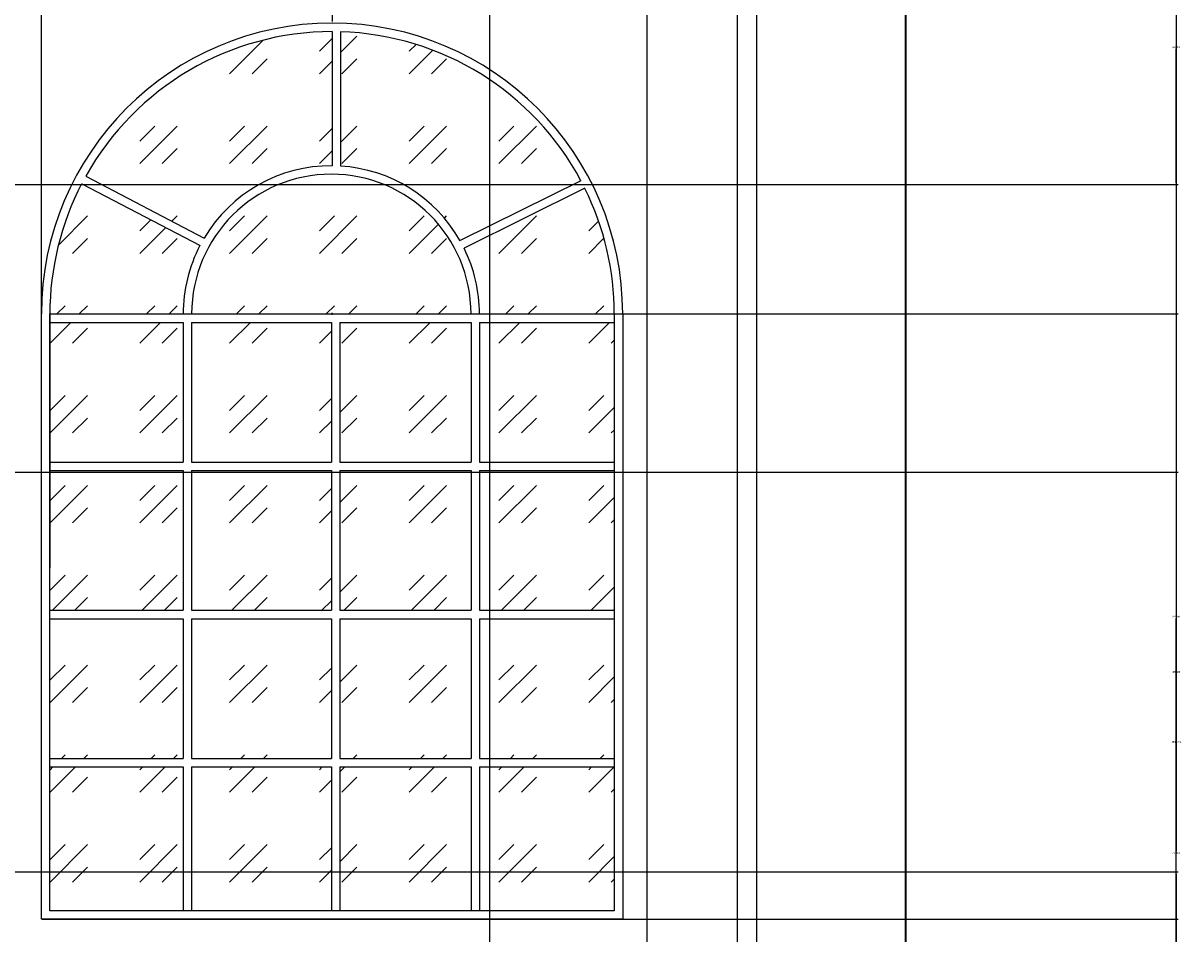
# Model space of a CAD drawing. Units: inches. Extents: x 93 to 565, y 123 to 656.
# Tile 12 of 18: x 456 to 565, y 377 to 463. Entities that reach past the tile are written whole.
import ezdxf

# ---------------------------------------------------------------- set-up
doc = ezdxf.new("R2010")
doc.units = ezdxf.units.IN
doc.header["$MEASUREMENT"] = 0
for name, color, linetype, lineweight in [('A-ANNO-DIMS', 2, 'Continuous', 18), ('A-ELEV', 7, 'Continuous', 35), ('A-GLAZ', 4, 'Continuous', 25)]:
    doc.layers.add(name, color=color, linetype=linetype, lineweight=lineweight)
doc.styles.get("Standard").update_dxf_attribs({"font": 'arial.ttf'})
doc.dimstyles.get("Standard").update_dxf_attribs({"dimtxt": 0.18, "dimasz": 0.18, "dimexe": 0.18, "dimexo": 0.0625, "dimgap": 0.09, "dimtad": 0, "dimtih": 1, "dimtoh": 1, "dimdec": 4, "dimzin": 0, "dimdsep": 46, "dimtxsty": 'Standard', "dimcen": 0.09, "dimadec": 0, "dimazin": 0, "dimtfac": 1, "dimtdec": 4, "dimtofl": 0, "dimtmove": 0, "dimatfit": 3, "dimfxl": 1, "dimtolj": 1, "dimtzin": 0, "dimarcsym": 0})

# ---------------------------------------------------------------- blocks, each defined once
blk = doc.blocks.new('WIN-ARCHED')
for p, q in [((26.67, 83.05), (26.67, 70.38)), ((27.47, 83.04), (27.47, 70.36)), ((3.39, 69.39), (14.58, 63.55)), ((50.18, 68.96), (38.77, 63.31)), ((3.01, 68.68), (14.19, 62.86)), ((50.55, 68.25), (39.15, 62.6)), ((0, 56.38), (12.6, 56.38)), ((0, 56.38), (0.2, 56.38)), ((0, 56.38), (0, 32.38)), ((13.4, 56.38), (39.8, 56.38)), ((40.6, 56.38), (53.33, 56.38)), ((0, 55.58), (12.6, 55.58)), ((12.6, 55.58), (12.6, 42.38)), ((13.4, 55.58), (13.4, 42.38)), ((13.4, 55.58), (26.6, 55.58)), ((26.6, 55.58), (26.6, 42.38)), ((27.4, 55.58), (27.4, 42.38)), ((27.4, 55.58), (39.8, 55.58)), ((39.8, 55.58), (39.8, 42.38)), ((40.6, 55.58), (40.6, 42.38)), ((40.6, 55.58), (53.33, 55.58)), ((0, 42.38), (12.6, 42.38)), ((0, 41.58), (12.6, 41.58)), ((12.6, 41.58), (12.6, 28.38)), ((13.4, 42.38), (26.6, 42.38)), ((13.4, 41.58), (13.4, 28.38)), ((13.4, 41.58), (26.6, 41.58)), ((26.6, 41.58), (26.6, 28.38)), ((27.4, 42.38), (39.8, 42.38)), ((27.4, 41.58), (27.4, 28.38)), ((27.4, 41.58), (39.8, 41.58)), ((39.8, 41.58), (39.8, 28.38)), ((40.6, 42.38), (53.33, 42.38)), ((40.6, 41.58), (40.6, 28.38)), ((40.6, 41.58), (53.33, 41.58)), ((0, 28.38), (12.6, 28.38)), ((0, 27.58), (12.6, 27.58)), ((12.6, 27.58), (12.6, 14.38)), ((13.4, 28.38), (26.6, 28.38)), ((13.4, 27.58), (13.4, 14.38)), ((13.4, 27.58), (26.6, 27.58)), ((26.6, 27.58), (26.6, 14.38)), ((27.4, 28.38), (39.8, 28.38)), ((27.4, 27.58), (27.4, 14.38)), ((27.4, 27.58), (39.8, 27.58)), ((39.8, 27.58), (39.8, 14.38)), ((40.6, 28.38), (53.33, 28.38)), ((40.6, 27.58), (40.6, 14.38)), ((40.6, 27.58), (53.33, 27.58)), ((0, 14.38), (12.6, 14.38)), ((13.4, 14.38), (26.6, 14.38)), ((27.4, 14.38), (39.8, 14.38)), ((40.6, 14.38), (53.33, 14.38)), ((0, 13.58), (12.6, 13.58)), ((12.6, 13.58), (12.6, 0)), ((13.4, 13.58), (13.4, 0)), ((13.4, 13.58), (26.6, 13.58)), ((26.6, 13.58), (26.6, 0)), ((27.4, 13.58), (27.4, 0)), ((27.4, 13.58), (39.8, 13.58)), ((39.8, 13.58), (39.8, 0)), ((40.6, 13.58), (40.6, 0)), ((40.6, 13.58), (53.33, 13.58))]:
    blk.add_line(p, q)
blk.add_lwpolyline([(53.33, 56.38), (53.33, 0), (0, 0), (0, 56.38)])
for centre, radius, start, end in [((26.67, 56.38), 26.67, 90, 150.8167), ((26.67, 56.38), 26.67, 28.1372, 88.2808), ((26.6, 56.38), 14, 89.7291, 149.1942), ((26.6, 56.38), 14, 29.6307, 86.4528), ((26.6, 56.38), 13.2, 0, 180), ((26.67, 56.38), 26.67, 152.5358, 180), ((26.67, 56.38), 26.67, 0, 26.418), ((26.6, 56.38), 14, 152.4701, 180), ((26.6, 56.38), 14, 0, 26.3549)]:
    blk.add_arc(centre, radius, start, end)
blk = doc.blocks.new('*D30')
at = {"layer": 'A-ANNO-DIMS', "color": 0, "lineweight": -2, "transparency": 16777216}
for p, q in [((437.19, 594.34), (437.19, 134)), ((539.08, 159.67), (539.08, 134)), ((437.37, 134.18), (487.75, 134.18)), ((538.9, 134.18), (488.52, 134.18))]:
    blk.add_line(p, q, dxfattribs=at)
at = {"layer": 'A-ANNO-DIMS', "color": 0, "transparency": 16777216}
for points in [[(437.37, 134.21), (437.37, 134.15), (437.19, 134.18)], [(538.9, 134.21), (538.9, 134.15), (539.08, 134.18)]]:
    blk.add_solid(points, dxfattribs=at)
at = {"layer": 'Defpoints', "color": 0, "transparency": 16777216}
for p in [(437.19, 594.4), (539.08, 159.73), (539.08, 134.18)]:
    blk.add_point(p, dxfattribs=at)
at = {"layer": 'A-ANNO-DIMS', "color": 0, "transparency": 16777216, "insert": (488.13, 134.18), "char_height": 0.18, "attachment_point": 5}
blk.add_mtext('\\A1;101.9', dxfattribs=at)
blk = doc.blocks.new('*D31')
at = {"layer": 'A-ANNO-DIMS', "color": 0, "lineweight": -2, "transparency": 16777216}
for p, q in [((417.87, 630.4), (564.81, 630.4)), ((564.63, 630.22), (564.63, 395.25)), ((564.63, 159.91), (564.63, 394.89)), ((119.14, 159.73), (564.81, 159.73))]:
    blk.add_line(p, q, dxfattribs=at)
at = {"layer": 'A-ANNO-DIMS', "color": 0, "transparency": 16777216}
for points in [[(564.6, 630.22), (564.66, 630.22), (564.63, 630.4)], [(564.6, 159.91), (564.66, 159.91), (564.63, 159.73)]]:
    blk.add_solid(points, dxfattribs=at)
at = {"layer": 'Defpoints', "color": 0, "transparency": 16777216}
for p in [(417.81, 630.4), (564.63, 630.4), (119.08, 159.73)]:
    blk.add_point(p, dxfattribs=at)
at = {"layer": 'A-ANNO-DIMS', "color": 0, "transparency": 16777216, "insert": (564.63, 395.07), "char_height": 0.18, "attachment_point": 5}
blk.add_mtext('\\A1;470.7', dxfattribs=at)
blk = doc.blocks.new('*D67')
at = {"layer": 'A-ANNO-DIMS', "color": 0, "lineweight": -2, "transparency": 16777216}
for p, q in [((331.87, 420.57), (564.81, 420.57)), ((564.63, 420.39), (564.63, 384.75)), ((564.63, 348.75), (564.63, 384.39)), ((331.87, 348.57), (564.81, 348.57))]:
    blk.add_line(p, q, dxfattribs=at)
at = {"layer": 'A-ANNO-DIMS', "color": 0, "transparency": 16777216}
for points in [[(564.6, 420.39), (564.66, 420.39), (564.63, 420.57)], [(564.6, 348.75), (564.66, 348.75), (564.63, 348.57)]]:
    blk.add_solid(points, dxfattribs=at)
at = {"layer": 'Defpoints', "color": 0, "transparency": 16777216}
for p in [(331.81, 420.57), (564.63, 420.57), (331.81, 348.57)]:
    blk.add_point(p, dxfattribs=at)
at = {"layer": 'A-ANNO-DIMS', "color": 0, "transparency": 16777216, "insert": (564.63, 384.57), "char_height": 0.18, "attachment_point": 5}
blk.add_mtext('\\A1;72', dxfattribs=at)
blk = doc.blocks.new('*D70')
at = {"layer": 'A-ANNO-DIMS', "color": 0, "lineweight": -2, "transparency": 16777216}
for p, q in [((428.68, 420.57), (564.81, 420.57)), ((564.63, 420.39), (564.63, 401.87)), ((564.63, 382.98), (564.63, 401.5)), ((428.68, 382.8), (564.81, 382.8))]:
    blk.add_line(p, q, dxfattribs=at)
at = {"layer": 'A-ANNO-DIMS', "color": 0, "transparency": 16777216}
for points in [[(564.6, 420.39), (564.66, 420.39), (564.63, 420.57)], [(564.6, 382.98), (564.66, 382.98), (564.63, 382.8)]]:
    blk.add_solid(points, dxfattribs=at)
at = {"layer": 'Defpoints', "color": 0, "transparency": 16777216}
for p in [(428.62, 420.57), (564.63, 420.57), (428.62, 382.8)]:
    blk.add_point(p, dxfattribs=at)
at = {"layer": 'A-ANNO-DIMS', "color": 0, "transparency": 16777216, "insert": (564.63, 401.68), "char_height": 0.18, "attachment_point": 5}
blk.add_mtext('\\A1;37.77', dxfattribs=at)
blk = doc.blocks.new('*D71')
at = {"layer": 'A-ANNO-DIMS', "color": 0, "lineweight": -2, "transparency": 16777216}
for p, q in [((428.68, 382.8), (564.81, 382.8)), ((564.63, 382.62), (564.63, 372.46)), ((564.63, 361.93), (564.63, 372.09)), ((437.25, 361.75), (564.81, 361.75))]:
    blk.add_line(p, q, dxfattribs=at)
at = {"layer": 'A-ANNO-DIMS', "color": 0, "transparency": 16777216}
for points in [[(564.6, 382.62), (564.66, 382.62), (564.63, 382.8)], [(564.6, 361.93), (564.66, 361.93), (564.63, 361.75)]]:
    blk.add_solid(points, dxfattribs=at)
at = {"layer": 'Defpoints', "color": 0, "transparency": 16777216}
for p in [(428.62, 382.8), (437.19, 361.75), (564.63, 361.75)]:
    blk.add_point(p, dxfattribs=at)
at = {"layer": 'A-ANNO-DIMS', "color": 0, "transparency": 16777216, "insert": (564.63, 372.27), "char_height": 0.18, "attachment_point": 5}
blk.add_mtext('\\A1;21.05', dxfattribs=at)
blk = doc.blocks.new('*D73')
at = {"layer": 'A-ANNO-DIMS', "color": 0, "lineweight": -2, "transparency": 16777216}
for p, q in [((437.25, 473.73), (564.81, 473.73)), ((564.63, 473.55), (564.63, 460.91)), ((564.63, 447.91), (564.63, 460.55)), ((437.25, 447.73), (564.81, 447.73))]:
    blk.add_line(p, q, dxfattribs=at)
at = {"layer": 'A-ANNO-DIMS', "color": 0, "transparency": 16777216}
for points in [[(564.6, 473.55), (564.66, 473.55), (564.63, 473.73)], [(564.6, 447.91), (564.66, 447.91), (564.63, 447.73)]]:
    blk.add_solid(points, dxfattribs=at)
at = {"layer": 'Defpoints', "color": 0, "transparency": 16777216}
for p in [(437.19, 473.73), (564.63, 473.73), (437.19, 447.73)]:
    blk.add_point(p, dxfattribs=at)
at = {"layer": 'A-ANNO-DIMS', "color": 0, "transparency": 16777216, "insert": (564.63, 460.73), "char_height": 0.18, "attachment_point": 5}
blk.add_mtext('\\A1;26', dxfattribs=at)
blk = doc.blocks.new('*D82')
at = {"layer": 'A-ANNO-DIMS', "color": 0, "lineweight": -2, "transparency": 16777216}
for p, q in [((437.19, 447.79), (437.19, 656.13)), ((437.37, 655.95), (446.83, 655.95)), ((457.21, 655.95), (447.76, 655.95)), ((457.39, 378.4), (457.39, 656.13))]:
    blk.add_line(p, q, dxfattribs=at)
at = {"layer": 'A-ANNO-DIMS', "color": 0, "transparency": 16777216}
for points in [[(437.37, 655.98), (437.37, 655.92), (437.19, 655.95)], [(457.21, 655.98), (457.21, 655.92), (457.39, 655.95)]]:
    blk.add_solid(points, dxfattribs=at)
at = {"layer": 'Defpoints', "color": 0, "transparency": 16777216}
for p in [(457.39, 655.95), (437.19, 447.73), (457.39, 378.34)]:
    blk.add_point(p, dxfattribs=at)
at = {"layer": 'A-ANNO-DIMS', "color": 0, "transparency": 16777216, "insert": (447.29, 655.95), "char_height": 0.18, "attachment_point": 5}
blk.add_mtext('\\A1;20.205', dxfattribs=at)
blk = doc.blocks.new('*D83')
at = {"layer": 'A-ANNO-DIMS', "color": 0, "lineweight": -2, "transparency": 16777216}
for p, q in [((457.46, 378.34), (564.81, 378.34)), ((564.63, 378.16), (564.63, 370.22)), ((564.63, 361.93), (564.63, 369.86)), ((437.25, 361.75), (564.81, 361.75))]:
    blk.add_line(p, q, dxfattribs=at)
at = {"layer": 'A-ANNO-DIMS', "color": 0, "transparency": 16777216}
for points in [[(564.6, 378.16), (564.66, 378.16), (564.63, 378.34)], [(564.6, 361.93), (564.66, 361.93), (564.63, 361.75)]]:
    blk.add_solid(points, dxfattribs=at)
at = {"layer": 'Defpoints', "color": 0, "transparency": 16777216}
for p in [(457.39, 378.34), (437.19, 361.75), (564.63, 361.75)]:
    blk.add_point(p, dxfattribs=at)
at = {"layer": 'A-ANNO-DIMS', "color": 0, "transparency": 16777216, "insert": (564.63, 370.04), "char_height": 0.18, "attachment_point": 5}
blk.add_mtext('\\A1;16.59', dxfattribs=at)
blk = doc.blocks.new('*D84')
at = {"layer": 'A-ANNO-DIMS', "color": 0, "lineweight": -2, "transparency": 16777216}
for p, q in [((458.26, 435.52), (564.81, 435.52)), ((564.63, 435.34), (564.63, 407.11)), ((564.63, 378.52), (564.63, 406.75)), ((457.46, 378.34), (564.81, 378.34))]:
    blk.add_line(p, q, dxfattribs=at)
at = {"layer": 'A-ANNO-DIMS', "color": 0, "transparency": 16777216}
for points in [[(564.6, 435.34), (564.66, 435.34), (564.63, 435.52)], [(564.6, 378.52), (564.66, 378.52), (564.63, 378.34)]]:
    blk.add_solid(points, dxfattribs=at)
at = {"layer": 'Defpoints', "color": 0, "transparency": 16777216}
for p in [(458.19, 435.52), (564.63, 435.52), (457.39, 378.34)]:
    blk.add_point(p, dxfattribs=at)
at = {"layer": 'A-ANNO-DIMS', "color": 0, "transparency": 16777216, "insert": (564.63, 406.93), "char_height": 0.18, "attachment_point": 5}
blk.add_mtext('\\A1;57.18', dxfattribs=at)
blk = doc.blocks.new('*D91')
at = {"layer": 'A-ANNO-DIMS', "color": 0, "lineweight": -2, "transparency": 16777216}
for p, q in [((499.73, 599.75), (499.73, 134)), ((437.19, 594.34), (437.19, 134)), ((437.37, 134.18), (468.07, 134.18)), ((499.55, 134.18), (468.85, 134.18))]:
    blk.add_line(p, q, dxfattribs=at)
at = {"layer": 'A-ANNO-DIMS', "color": 0, "transparency": 16777216}
for points in [[(437.37, 134.21), (437.37, 134.15), (437.19, 134.18)], [(499.55, 134.21), (499.55, 134.15), (499.73, 134.18)]]:
    blk.add_solid(points, dxfattribs=at)
at = {"layer": 'Defpoints', "color": 0, "transparency": 16777216}
for p in [(499.73, 599.82), (437.19, 594.4), (499.73, 134.18)]:
    blk.add_point(p, dxfattribs=at)
at = {"layer": 'A-ANNO-DIMS', "color": 0, "transparency": 16777216, "insert": (468.46, 134.18), "char_height": 0.18, "attachment_point": 5}
blk.add_mtext('\\A1;62.54', dxfattribs=at)
blk = doc.blocks.new('*D92')
at = {"layer": 'A-ANNO-DIMS', "color": 0, "lineweight": -2, "transparency": 16777216}
for p, q in [((523.14, 603.14), (523.14, 134)), ((499.73, 599.75), (499.73, 134)), ((499.91, 134.18), (510.97, 134.18)), ((522.96, 134.18), (511.9, 134.18))]:
    blk.add_line(p, q, dxfattribs=at)
at = {"layer": 'A-ANNO-DIMS', "color": 0, "transparency": 16777216}
for points in [[(499.91, 134.21), (499.91, 134.15), (499.73, 134.18)], [(522.96, 134.21), (522.96, 134.15), (523.14, 134.18)]]:
    blk.add_solid(points, dxfattribs=at)
at = {"layer": 'Defpoints', "color": 0, "transparency": 16777216}
for p in [(523.14, 603.2), (499.73, 599.82), (523.14, 134.18)]:
    blk.add_point(p, dxfattribs=at)
at = {"layer": 'A-ANNO-DIMS', "color": 0, "transparency": 16777216, "insert": (511.44, 134.18), "char_height": 0.18, "attachment_point": 5}
blk.add_mtext('\\A1;23.412', dxfattribs=at)
blk = doc.blocks.new('*D93')
at = {"layer": 'A-ANNO-DIMS', "color": 0, "lineweight": -2, "transparency": 16777216}
for p, q in [((523.14, 603.14), (523.14, 134)), ((539.08, 594.34), (539.08, 134)), ((523.32, 134.18), (530.66, 134.18)), ((538.9, 134.18), (531.57, 134.18))]:
    blk.add_line(p, q, dxfattribs=at)
at = {"layer": 'A-ANNO-DIMS', "color": 0, "transparency": 16777216}
for points in [[(523.32, 134.21), (523.32, 134.15), (523.14, 134.18)], [(538.9, 134.21), (538.9, 134.15), (539.08, 134.18)]]:
    blk.add_solid(points, dxfattribs=at)
at = {"layer": 'Defpoints', "color": 0, "transparency": 16777216}
for p in [(523.14, 603.2), (539.08, 594.4), (539.08, 134.18)]:
    blk.add_point(p, dxfattribs=at)
at = {"layer": 'A-ANNO-DIMS', "color": 0, "transparency": 16777216, "insert": (531.11, 134.18), "char_height": 0.18, "attachment_point": 5}
blk.add_mtext('\\A1;15.938', dxfattribs=at)
blk = doc.blocks.new('*D101')
at = {"layer": 'A-ANNO-DIMS', "color": 0, "lineweight": -2, "transparency": 16777216}
for p, q in [((485.04, 479.47), (484.86, 479.47)), ((484.86, 479.47), (484.86, 463.17)), ((484.77, 435.52), (484.95, 435.52)), ((484.86, 435.43), (484.86, 435.61))]:
    blk.add_line(p, q, dxfattribs=at)
at = {"layer": 'A-ANNO-DIMS', "color": 0, "transparency": 16777216}
blk.add_solid([(484.83, 463.17), (484.89, 463.17), (484.86, 462.99)], dxfattribs=at)
at = {"layer": 'Defpoints', "color": 0, "transparency": 16777216}
for p in [(484.86, 462.99), (484.86, 435.52)]:
    blk.add_point(p, dxfattribs=at)
at = {"layer": 'A-ANNO-DIMS', "color": 0, "transparency": 16777216, "insert": (485.78, 479.47), "char_height": 0.18, "attachment_point": 5}
blk.add_mtext('\\A1;2X R27.466', dxfattribs=at)
blk = doc.blocks.new('*D109')
at = {"layer": 'A-ANNO-DIMS', "color": 0, "lineweight": -2, "transparency": 16777216}
for p, q in [((437.19, 594.34), (437.19, 134)), ((539.08, 159.67), (539.08, 134)), ((437.37, 134.18), (487.63, 134.18)), ((538.9, 134.18), (488.64, 134.18))]:
    blk.add_line(p, q, dxfattribs=at)
at = {"layer": 'A-ANNO-DIMS', "color": 0, "transparency": 16777216}
for points in [[(437.37, 134.21), (437.37, 134.15), (437.19, 134.18)], [(538.9, 134.21), (538.9, 134.15), (539.08, 134.18)]]:
    blk.add_solid(points, dxfattribs=at)
at = {"layer": 'Defpoints', "color": 0, "transparency": 16777216}
for p in [(437.19, 594.4), (539.08, 159.73), (539.08, 134.18)]:
    blk.add_point(p, dxfattribs=at)
at = {"layer": 'A-ANNO-DIMS', "color": 0, "transparency": 16777216, "insert": (488.13, 134.18), "char_height": 0.18, "attachment_point": 5}
blk.add_mtext('\\A1;101.891', dxfattribs=at)
blk = doc.blocks.new('*D110')
at = {"layer": 'A-ANNO-DIMS', "color": 0, "lineweight": -2, "transparency": 16777216}
for p, q in [((417.87, 630.4), (564.81, 630.4)), ((564.63, 630.22), (564.63, 395.25)), ((564.63, 159.91), (564.63, 394.89)), ((119.14, 159.73), (564.81, 159.73))]:
    blk.add_line(p, q, dxfattribs=at)
at = {"layer": 'A-ANNO-DIMS', "color": 0, "transparency": 16777216}
for points in [[(564.6, 630.22), (564.66, 630.22), (564.63, 630.4)], [(564.6, 159.91), (564.66, 159.91), (564.63, 159.73)]]:
    blk.add_solid(points, dxfattribs=at)
at = {"layer": 'Defpoints', "color": 0, "transparency": 16777216}
for p in [(417.81, 630.4), (564.63, 630.4), (119.08, 159.73)]:
    blk.add_point(p, dxfattribs=at)
at = {"layer": 'A-ANNO-DIMS', "color": 0, "transparency": 16777216, "insert": (564.63, 395.07), "char_height": 0.18, "attachment_point": 5}
blk.add_mtext('\\A1;470.673', dxfattribs=at)
blk = doc.blocks.new('*D146')
at = {"layer": 'A-ANNO-DIMS', "color": 0, "lineweight": -2, "transparency": 16777216}
for p, q in [((331.87, 420.57), (564.81, 420.57)), ((564.63, 420.39), (564.63, 384.75)), ((564.63, 348.75), (564.63, 384.39)), ((331.87, 348.57), (564.81, 348.57))]:
    blk.add_line(p, q, dxfattribs=at)
at = {"layer": 'A-ANNO-DIMS', "color": 0, "transparency": 16777216}
for points in [[(564.6, 420.39), (564.66, 420.39), (564.63, 420.57)], [(564.6, 348.75), (564.66, 348.75), (564.63, 348.57)]]:
    blk.add_solid(points, dxfattribs=at)
at = {"layer": 'Defpoints', "color": 0, "transparency": 16777216}
for p in [(331.81, 420.57), (564.63, 420.57), (331.81, 348.57)]:
    blk.add_point(p, dxfattribs=at)
at = {"layer": 'A-ANNO-DIMS', "color": 0, "transparency": 16777216, "insert": (564.63, 384.57), "char_height": 0.18, "attachment_point": 5}
blk.add_mtext('\\A1;72.000', dxfattribs=at)
blk = doc.blocks.new('*D149')
at = {"layer": 'A-ANNO-DIMS', "color": 0, "lineweight": -2, "transparency": 16777216}
for p, q in [((428.68, 420.57), (564.81, 420.57)), ((564.63, 420.39), (564.63, 401.87)), ((564.63, 382.98), (564.63, 401.5)), ((428.68, 382.8), (564.81, 382.8))]:
    blk.add_line(p, q, dxfattribs=at)
at = {"layer": 'A-ANNO-DIMS', "color": 0, "transparency": 16777216}
for points in [[(564.6, 420.39), (564.66, 420.39), (564.63, 420.57)], [(564.6, 382.98), (564.66, 382.98), (564.63, 382.8)]]:
    blk.add_solid(points, dxfattribs=at)
at = {"layer": 'Defpoints', "color": 0, "transparency": 16777216}
for p in [(428.62, 420.57), (564.63, 420.57), (428.62, 382.8)]:
    blk.add_point(p, dxfattribs=at)
at = {"layer": 'A-ANNO-DIMS', "color": 0, "transparency": 16777216, "insert": (564.63, 401.68), "char_height": 0.18, "attachment_point": 5}
blk.add_mtext('\\A1;37.768', dxfattribs=at)
blk = doc.blocks.new('*D150')
at = {"layer": 'A-ANNO-DIMS', "color": 0, "lineweight": -2, "transparency": 16777216}
for p, q in [((428.68, 382.8), (564.81, 382.8)), ((564.63, 382.62), (564.63, 372.46)), ((564.63, 361.93), (564.63, 372.09)), ((437.25, 361.75), (564.81, 361.75))]:
    blk.add_line(p, q, dxfattribs=at)
at = {"layer": 'A-ANNO-DIMS', "color": 0, "transparency": 16777216}
for points in [[(564.6, 382.62), (564.66, 382.62), (564.63, 382.8)], [(564.6, 361.93), (564.66, 361.93), (564.63, 361.75)]]:
    blk.add_solid(points, dxfattribs=at)
at = {"layer": 'Defpoints', "color": 0, "transparency": 16777216}
for p in [(428.62, 382.8), (437.19, 361.75), (564.63, 361.75)]:
    blk.add_point(p, dxfattribs=at)
at = {"layer": 'A-ANNO-DIMS', "color": 0, "transparency": 16777216, "insert": (564.63, 372.27), "char_height": 0.18, "attachment_point": 5}
blk.add_mtext('\\A1;21.052', dxfattribs=at)
blk = doc.blocks.new('*D152')
at = {"layer": 'A-ANNO-DIMS', "color": 0, "lineweight": -2, "transparency": 16777216}
for p, q in [((437.25, 473.73), (564.81, 473.73)), ((564.63, 473.55), (564.63, 460.91)), ((564.63, 447.91), (564.63, 460.55)), ((437.25, 447.73), (564.81, 447.73))]:
    blk.add_line(p, q, dxfattribs=at)
at = {"layer": 'A-ANNO-DIMS', "color": 0, "transparency": 16777216}
for points in [[(564.6, 473.55), (564.66, 473.55), (564.63, 473.73)], [(564.6, 447.91), (564.66, 447.91), (564.63, 447.73)]]:
    blk.add_solid(points, dxfattribs=at)
at = {"layer": 'Defpoints', "color": 0, "transparency": 16777216}
for p in [(437.19, 473.73), (564.63, 473.73), (437.19, 447.73)]:
    blk.add_point(p, dxfattribs=at)
at = {"layer": 'A-ANNO-DIMS', "color": 0, "transparency": 16777216, "insert": (564.63, 460.73), "char_height": 0.18, "attachment_point": 5}
blk.add_mtext('\\A1;26.000', dxfattribs=at)
blk = doc.blocks.new('*D161')
at = {"layer": 'A-ANNO-DIMS', "color": 0, "lineweight": -2, "transparency": 16777216}
for p, q in [((437.19, 447.79), (437.19, 656.13)), ((437.37, 655.95), (446.83, 655.95)), ((457.21, 655.95), (447.76, 655.95)), ((457.39, 378.4), (457.39, 656.13))]:
    blk.add_line(p, q, dxfattribs=at)
at = {"layer": 'A-ANNO-DIMS', "color": 0, "transparency": 16777216}
for points in [[(437.37, 655.98), (437.37, 655.92), (437.19, 655.95)], [(457.21, 655.98), (457.21, 655.92), (457.39, 655.95)]]:
    blk.add_solid(points, dxfattribs=at)
at = {"layer": 'Defpoints', "color": 0, "transparency": 16777216}
for p in [(457.39, 655.95), (437.19, 447.73), (457.39, 378.34)]:
    blk.add_point(p, dxfattribs=at)
at = {"layer": 'A-ANNO-DIMS', "color": 0, "transparency": 16777216, "insert": (447.29, 655.95), "char_height": 0.18, "attachment_point": 5}
blk.add_mtext('\\A1;20.205', dxfattribs=at)
blk = doc.blocks.new('*D162')
at = {"layer": 'A-ANNO-DIMS', "color": 0, "lineweight": -2, "transparency": 16777216}
for p, q in [((457.46, 378.34), (564.81, 378.34)), ((564.63, 378.16), (564.63, 370.22)), ((564.63, 361.93), (564.63, 369.86)), ((437.25, 361.75), (564.81, 361.75))]:
    blk.add_line(p, q, dxfattribs=at)
at = {"layer": 'A-ANNO-DIMS', "color": 0, "transparency": 16777216}
for points in [[(564.6, 378.16), (564.66, 378.16), (564.63, 378.34)], [(564.6, 361.93), (564.66, 361.93), (564.63, 361.75)]]:
    blk.add_solid(points, dxfattribs=at)
at = {"layer": 'Defpoints', "color": 0, "transparency": 16777216}
for p in [(457.39, 378.34), (437.19, 361.75), (564.63, 361.75)]:
    blk.add_point(p, dxfattribs=at)
at = {"layer": 'A-ANNO-DIMS', "color": 0, "transparency": 16777216, "insert": (564.63, 370.04), "char_height": 0.18, "attachment_point": 5}
blk.add_mtext('\\A1;16.590', dxfattribs=at)
blk = doc.blocks.new('*D163')
at = {"layer": 'A-ANNO-DIMS', "color": 0, "lineweight": -2, "transparency": 16777216}
for p, q in [((458.26, 435.52), (564.81, 435.52)), ((564.63, 435.34), (564.63, 407.11)), ((564.63, 378.52), (564.63, 406.75)), ((457.46, 378.34), (564.81, 378.34))]:
    blk.add_line(p, q, dxfattribs=at)
at = {"layer": 'A-ANNO-DIMS', "color": 0, "transparency": 16777216}
for points in [[(564.6, 435.34), (564.66, 435.34), (564.63, 435.52)], [(564.6, 378.52), (564.66, 378.52), (564.63, 378.34)]]:
    blk.add_solid(points, dxfattribs=at)
at = {"layer": 'Defpoints', "color": 0, "transparency": 16777216}
for p in [(458.19, 435.52), (564.63, 435.52), (457.39, 378.34)]:
    blk.add_point(p, dxfattribs=at)
at = {"layer": 'A-ANNO-DIMS', "color": 0, "transparency": 16777216, "insert": (564.63, 406.93), "char_height": 0.18, "attachment_point": 5}
blk.add_mtext('\\A1;57.184', dxfattribs=at)
blk = doc.blocks.new('*D170')
at = {"layer": 'A-ANNO-DIMS', "color": 0, "lineweight": -2, "transparency": 16777216}
for p, q in [((499.73, 599.75), (499.73, 134)), ((437.19, 594.34), (437.19, 134)), ((437.37, 134.18), (468.01, 134.18)), ((499.55, 134.18), (468.91, 134.18))]:
    blk.add_line(p, q, dxfattribs=at)
at = {"layer": 'A-ANNO-DIMS', "color": 0, "transparency": 16777216}
for points in [[(437.37, 134.21), (437.37, 134.15), (437.19, 134.18)], [(499.55, 134.21), (499.55, 134.15), (499.73, 134.18)]]:
    blk.add_solid(points, dxfattribs=at)
at = {"layer": 'Defpoints', "color": 0, "transparency": 16777216}
for p in [(499.73, 599.82), (437.19, 594.4), (499.73, 134.18)]:
    blk.add_point(p, dxfattribs=at)
at = {"layer": 'A-ANNO-DIMS', "color": 0, "transparency": 16777216, "insert": (468.46, 134.18), "char_height": 0.18, "attachment_point": 5}
blk.add_mtext('\\A1;62.541', dxfattribs=at)
blk = doc.blocks.new('*D171')
at = {"layer": 'A-ANNO-DIMS', "color": 0, "lineweight": -2, "transparency": 16777216}
for p, q in [((523.14, 603.14), (523.14, 134)), ((499.73, 599.75), (499.73, 134)), ((499.91, 134.18), (510.97, 134.18)), ((522.96, 134.18), (511.9, 134.18))]:
    blk.add_line(p, q, dxfattribs=at)
at = {"layer": 'A-ANNO-DIMS', "color": 0, "transparency": 16777216}
for points in [[(499.91, 134.21), (499.91, 134.15), (499.73, 134.18)], [(522.96, 134.21), (522.96, 134.15), (523.14, 134.18)]]:
    blk.add_solid(points, dxfattribs=at)
at = {"layer": 'Defpoints', "color": 0, "transparency": 16777216}
for p in [(523.14, 603.2), (499.73, 599.82), (523.14, 134.18)]:
    blk.add_point(p, dxfattribs=at)
at = {"layer": 'A-ANNO-DIMS', "color": 0, "transparency": 16777216, "insert": (511.44, 134.18), "char_height": 0.18, "attachment_point": 5}
blk.add_mtext('\\A1;23.412', dxfattribs=at)
blk = doc.blocks.new('*D172')
at = {"layer": 'A-ANNO-DIMS', "color": 0, "lineweight": -2, "transparency": 16777216}
for p, q in [((523.14, 603.14), (523.14, 134)), ((539.08, 594.34), (539.08, 134)), ((523.32, 134.18), (530.66, 134.18)), ((538.9, 134.18), (531.57, 134.18))]:
    blk.add_line(p, q, dxfattribs=at)
at = {"layer": 'A-ANNO-DIMS', "color": 0, "transparency": 16777216}
for points in [[(523.32, 134.21), (523.32, 134.15), (523.14, 134.18)], [(538.9, 134.21), (538.9, 134.15), (539.08, 134.18)]]:
    blk.add_solid(points, dxfattribs=at)
at = {"layer": 'Defpoints', "color": 0, "transparency": 16777216}
for p in [(523.14, 603.2), (539.08, 594.4), (539.08, 134.18)]:
    blk.add_point(p, dxfattribs=at)
at = {"layer": 'A-ANNO-DIMS', "color": 0, "transparency": 16777216, "insert": (531.11, 134.18), "char_height": 0.18, "attachment_point": 5}
blk.add_mtext('\\A1;15.938', dxfattribs=at)
blk = doc.blocks.new('*D185')
at = {"layer": 'A-ANNO-DIMS', "color": 0, "lineweight": -2, "transparency": 16777216}
for p, q in [((514.64, 358.44), (514.64, 656.13)), ((514.82, 655.95), (519.36, 655.95)), ((524.81, 655.95), (520.27, 655.95)), ((524.99, 363.79), (524.99, 656.13))]:
    blk.add_line(p, q, dxfattribs=at)
at = {"layer": 'A-ANNO-DIMS', "color": 0, "transparency": 16777216}
for points in [[(514.82, 655.98), (514.82, 655.92), (514.64, 655.95)], [(524.81, 655.98), (524.81, 655.92), (524.99, 655.95)]]:
    blk.add_solid(points, dxfattribs=at)
at = {"layer": 'Defpoints', "color": 0, "transparency": 16777216}
for p in [(524.99, 655.95), (524.99, 363.73), (514.64, 358.37)]:
    blk.add_point(p, dxfattribs=at)
at = {"layer": 'A-ANNO-DIMS', "color": 0, "transparency": 16777216, "insert": (519.81, 655.95), "char_height": 0.18, "attachment_point": 5}
blk.add_mtext('\\A1;10.344', dxfattribs=at)
blk = doc.blocks.new('*D186')
at = {"layer": 'A-ANNO-DIMS', "color": 0, "lineweight": -2, "transparency": 16777216}
for p, q in [((524.99, 363.79), (524.99, 656.13)), ((525.17, 655.95), (531.58, 655.95)), ((538.9, 655.95), (532.49, 655.95)), ((539.08, 363.79), (539.08, 656.13))]:
    blk.add_line(p, q, dxfattribs=at)
at = {"layer": 'A-ANNO-DIMS', "color": 0, "transparency": 16777216}
for points in [[(525.17, 655.98), (525.17, 655.92), (524.99, 655.95)], [(538.9, 655.98), (538.9, 655.92), (539.08, 655.95)]]:
    blk.add_solid(points, dxfattribs=at)
at = {"layer": 'Defpoints', "color": 0, "transparency": 16777216}
for p in [(539.08, 655.95), (524.99, 363.73), (539.08, 363.73)]:
    blk.add_point(p, dxfattribs=at)
at = {"layer": 'A-ANNO-DIMS', "color": 0, "transparency": 16777216, "insert": (532.03, 655.95), "char_height": 0.18, "attachment_point": 5}
blk.add_mtext('\\A1;14.093', dxfattribs=at)
blk = doc.blocks.new('*D199')
at = {"layer": 'A-ANNO-DIMS', "color": 0, "lineweight": -2, "transparency": 16777216}
for p, q in [((485.04, 479.47), (484.86, 479.47)), ((484.86, 479.47), (484.86, 463.17)), ((484.77, 435.52), (484.95, 435.52)), ((484.86, 435.43), (484.86, 435.61))]:
    blk.add_line(p, q, dxfattribs=at)
at = {"layer": 'A-ANNO-DIMS', "color": 0, "transparency": 16777216}
blk.add_solid([(484.83, 463.17), (484.89, 463.17), (484.86, 462.99)], dxfattribs=at)
at = {"layer": 'Defpoints', "color": 0, "transparency": 16777216}
for p in [(484.86, 462.99), (484.86, 435.52)]:
    blk.add_point(p, dxfattribs=at)
at = {"layer": 'A-ANNO-DIMS', "color": 0, "transparency": 16777216, "insert": (485.78, 479.47), "char_height": 0.18, "attachment_point": 5}
blk.add_mtext('\\A1;2X R27.466', dxfattribs=at)

msp = doc.modelspace()

# ---------------------------------------------------------------- hatches: boundary and pattern name
at = {"layer": 'A-GLAZ'}
h = msp.add_hatch(dxfattribs=at)
h.set_pattern_fill('GOST_GLASS', color=256)
h.set_pattern_definition([(45, (0, 0), (8.48528, 0), [5, -7]), (45, (2.1213, 0), (8.48528, 0), [2, -10]), (45, (0, 2.1213), (8.48528, 0), [2, -10])])
h.paths.add_polyline_path([(484.8595, 462.1876, 0.27177204), (461.5782, 448.524), (472.7686, 442.6912, -0.26544926), (484.8595, 449.5212)])
h.paths.add_polyline_path([(485.6595, 462.1756), (485.6595, 449.4946, -0.25314153), (496.9625, 442.4431), (508.3743, 448.0968, 0.268621)])
h.paths.add_polyline_path([(508.741, 447.3856), (497.3382, 441.7364, -0.11550447), (498.7933, 435.5214), (511.5257, 435.5214, 0.11578361)])
h.paths.add_polyline_path([(511.5257, 434.7214), (498.7933, 434.7214), (498.7933, 421.5214), (511.5257, 421.5214)])
h.paths.add_polyline_path([(497.9933, 434.7214), (485.5933, 434.7214), (485.5933, 421.5214), (497.9933, 421.5214)])
h.paths.add_polyline_path([(484.7933, 434.7214), (471.5933, 434.7214), (471.5933, 421.5214), (484.7933, 421.5214)])
h.paths.add_polyline_path([(470.7933, 434.7214), (458.1933, 434.7214), (458.1933, 421.5214), (470.7933, 421.5214)])
h.paths.add_polyline_path([(472.3785, 441.9924), (461.1986, 447.8197, 0.12041216), (458.1933, 435.5214), (458.3933, 435.5214), (470.7933, 435.5214, -0.12070313)])
h.paths.add_polyline_path([(471.5933, 435.5214), (497.9933, 435.5214, 1)])
h.paths.add_polyline_path([(470.7933, 420.7214), (458.1933, 420.7214), (458.1933, 411.5214), (458.1933, 407.5214), (470.7933, 407.5214)])
h.paths.add_polyline_path([(484.7933, 420.7214), (471.5933, 420.7214), (471.5933, 407.5214), (484.7933, 407.5214)])
h.paths.add_polyline_path([(497.9933, 420.7214), (485.5933, 420.7214), (485.5933, 407.5214), (497.9933, 407.5214)])
h.paths.add_polyline_path([(511.5257, 420.7214), (498.7933, 420.7214), (498.7933, 407.5214), (511.5257, 407.5214)])
h.paths.add_polyline_path([(511.5257, 406.7214), (498.7933, 406.7214), (498.7933, 393.5214), (511.5257, 393.5214)])
h.paths.add_polyline_path([(511.5257, 392.7214), (498.7933, 392.7214), (498.7933, 379.1372), (511.5257, 379.1372)])
h.paths.add_polyline_path([(497.9933, 392.7214), (485.5933, 392.7214), (485.5933, 379.1372), (497.9933, 379.1372)])
h.paths.add_polyline_path([(497.9933, 406.7214), (485.5933, 406.7214), (485.5933, 393.5214), (497.9933, 393.5214)])
h.paths.add_polyline_path([(484.7933, 406.7214), (471.5933, 406.7214), (471.5933, 393.5214), (484.7933, 393.5214)])
h.paths.add_polyline_path([(484.7933, 392.7214), (471.5933, 392.7214), (471.5933, 379.1372), (484.7933, 379.1372)])
h.paths.add_polyline_path([(470.7933, 392.7214), (458.1933, 392.7214), (458.1933, 379.1372), (470.7933, 379.1372)])
h.paths.add_polyline_path([(470.7933, 406.7214), (458.1933, 406.7214), (458.1933, 393.5214), (470.7933, 393.5214)])

# ---------------------------------------------------------------- linework, layer by layer
at = {"layer": 'A-ELEV'}
msp.add_line((539.0794, 363.7323), (539.0794, 594.4048), dxfattribs=at)
at = {"layer": 'A-GLAZ'}
for p, q in [((485.6595, 462.9876), (485.6595, 462.9759)), ((460.859, 448.8989), (460.8685, 448.8939)), ((509.1027, 448.4576), (509.0915, 448.4521))]:
    msp.add_line(p, q, dxfattribs=at)
msp.add_lwpolyline([(512.3257, 435.5214), (512.3257, 378.3372), (457.3933, 378.3372), (457.3933, 435.5214)], dxfattribs=at)
msp.add_arc((484.8595, 435.5214), 27.4662, 0, 180, dxfattribs=at)

# ---------------------------------------------------------------- block references
msp.add_blockref('WIN-ARCHED', (458.193, 379.137), dxfattribs=at)

# ---------------------------------------------------------------- dimensions: what is measured, and where the dimension line sits
at = {"layer": 'A-ANNO-DIMS'}
for base, p1, p2, override, picture, middle in [((457.3933, 655.9548), (437.1885, 447.7323), (457.3933, 378.3372), {"dimdec": 3, "dimlfac": 1, "dimrnd": 0, "dimzin": 0, "dimdsep": 46, "dimlunit": 2}, '*D82', (447.2909, 655.9548)), ((457.3933, 655.9548), (437.1885, 447.7323), (457.3933, 378.3372), {"dimdec": 3, "dimlfac": 1, "dimrnd": 0, "dimzin": 0, "dimdsep": 46, "dimlunit": 2}, '*D161', (447.2909, 655.9548)), ((524.9864, 655.9548), (514.6424, 358.3735), (524.9864, 363.7323), {"dimdec": 3, "dimlfac": 1, "dimrnd": 0, "dimzin": 0, "dimdsep": 46, "dimlunit": 2}, '*D185', (519.8144, 655.9548)), ((539.0794, 655.9548), (524.9864, 363.7323), (539.0794, 363.7323), {"dimdec": 3, "dimlfac": 1, "dimrnd": 0, "dimzin": 0, "dimdsep": 46, "dimlunit": 2}, '*D186', (532.0329, 655.9548)), ((523.1415, 134.1823), (499.7291, 599.8171), (523.1415, 603.1979), {"dimdec": 3, "dimlfac": 1, "dimrnd": 0, "dimzin": 0, "dimdsep": 46, "dimlunit": 2}, '*D92', (511.4353, 134.1823)), ((523.1415, 134.1823), (499.7291, 599.8171), (523.1415, 603.1979), {"dimdec": 3, "dimlfac": 1, "dimrnd": 0, "dimzin": 0, "dimdsep": 46, "dimlunit": 2}, '*D171', (511.4353, 134.1823)), ((539.0794, 134.1823), (523.1415, 603.1979), (539.0794, 594.4048), {"dimdec": 3, "dimlfac": 1, "dimrnd": 0, "dimzin": 0, "dimdsep": 46, "dimlunit": 2}, '*D93', (531.1104, 134.1823)), ((539.0794, 134.1823), (523.1415, 603.1979), (539.0794, 594.4048), {"dimdec": 3, "dimlfac": 1, "dimrnd": 0, "dimzin": 0, "dimdsep": 46, "dimlunit": 2}, '*D172', (531.1104, 134.1823)), ((499.7291, 134.1823), (437.1885, 594.4048), (499.7291, 599.8171), {"dimdec": 2, "dimlfac": 1, "dimrnd": 0, "dimzin": 0, "dimdsep": 46, "dimlunit": 2}, '*D91', (468.4588, 134.1823)), ((499.7291, 134.1823), (437.1885, 594.4048), (499.7291, 599.8171), {"dimdec": 3, "dimlfac": 1, "dimrnd": 0, "dimzin": 0, "dimdsep": 46, "dimlunit": 2}, '*D170', (468.4588, 134.1823)), ((539.0794, 134.1823), (437.1885, 594.4048), (539.0794, 159.7323), {"dimdec": 1, "dimlfac": 1, "dimrnd": 0, "dimzin": 0, "dimdsep": 46, "dimlunit": 2}, '*D30', (488.1339, 134.1823)), ((539.0794, 134.1823), (437.1885, 594.4048), (539.0794, 159.7323), {"dimdec": 3, "dimlfac": 1, "dimrnd": 0, "dimzin": 0, "dimdsep": 46, "dimlunit": 2}, '*D109', (488.1339, 134.1823))]:
    dim = msp.add_linear_dim(base=base, p1=p1, p2=p2, dimstyle='Standard', override=override, dxfattribs=at)
    dim.commit()
    dim.dimension.update_dxf_attribs({"geometry": picture, "text_midpoint": middle})
for base, p1, p2, override, picture, middle in [((564.6294, 630.4048), (119.0794, 159.7323), (417.8097, 630.4048), {"dimdec": 1, "dimlfac": 1, "dimrnd": 0, "dimzin": 0, "dimdsep": 46, "dimlunit": 2}, '*D31', (564.6294, 395.0685)), ((564.62936, 630.40478), (119.07936, 159.73225), (417.80971, 630.40477), {"dimdec": 3, "dimlfac": 1, "dimrnd": 0, "dimzin": 0, "dimdsep": 46, "dimlunit": 2}, '*D110', (564.62936, 395.06851)), ((564.6294, 473.7323), (437.1885, 447.7323), (437.1885, 473.7323), {"dimdec": 0, "dimlfac": 1, "dimrnd": 0, "dimzin": 0, "dimdsep": 46, "dimlunit": 2}, '*D73', (564.6294, 460.7323)), ((564.6294, 473.7323), (437.1885, 447.7323), (437.1885, 473.7323), {"dimdec": 3, "dimlfac": 1, "dimrnd": 0, "dimzin": 0, "dimdsep": 46, "dimlunit": 2}, '*D152', (564.6294, 460.7323)), ((564.6294, 435.5214), (457.3933, 378.3372), (458.1933, 435.5214), {"dimdec": 2, "dimlfac": 1, "dimrnd": 0, "dimzin": 0, "dimdsep": 46, "dimlunit": 2}, '*D84', (564.6294, 406.9293)), ((564.6294, 435.5214), (457.3933, 378.3372), (458.1933, 435.5214), {"dimdec": 3, "dimlfac": 1, "dimrnd": 0, "dimzin": 0, "dimdsep": 46, "dimlunit": 2}, '*D163', (564.6294, 406.9293)), ((564.6294, 420.5674), (331.8112, 348.5674), (331.8112, 420.5674), {"dimdec": 0, "dimlfac": 1, "dimrnd": 0, "dimzin": 0, "dimdsep": 46, "dimlunit": 2}, '*D67', (564.6294, 384.5674)), ((564.6294, 420.5674), (331.8112, 348.5674), (331.8112, 420.5674), {"dimdec": 3, "dimlfac": 1, "dimrnd": 0, "dimzin": 0, "dimdsep": 46, "dimlunit": 2}, '*D146', (564.6294, 384.5674)), ((564.6294, 420.5674), (428.6158, 382.7996), (428.6158, 420.5674), {"dimdec": 2, "dimlfac": 1, "dimrnd": 0, "dimzin": 0, "dimdsep": 46, "dimlunit": 2}, '*D70', (564.6294, 401.6835)), ((564.6294, 420.5674), (428.6158, 382.7996), (428.6158, 420.5674), {"dimdec": 3, "dimlfac": 1, "dimrnd": 0, "dimzin": 0, "dimdsep": 46, "dimlunit": 2}, '*D149', (564.6294, 401.6835)), ((564.6294, 361.7477), (428.6158, 382.7996), (437.1885, 361.7477), {"dimdec": 2, "dimlfac": 1, "dimrnd": 0, "dimzin": 0, "dimdsep": 46, "dimlunit": 2}, '*D71', (564.6294, 372.2736)), ((564.6294, 361.7477), (428.6158, 382.7996), (437.1885, 361.7477), {"dimdec": 3, "dimlfac": 1, "dimrnd": 0, "dimzin": 0, "dimdsep": 46, "dimlunit": 2}, '*D150', (564.6294, 372.2736)), ((564.6294, 361.7477), (457.3933, 378.3372), (437.1885, 361.7477), {"dimdec": 2, "dimlfac": 1, "dimrnd": 0, "dimzin": 0, "dimdsep": 46, "dimlunit": 2}, '*D83', (564.6294, 370.0424)), ((564.62936, 361.74766), (457.3933, 378.33724), (437.18851, 361.74766), {"dimdec": 3, "dimlfac": 1, "dimrnd": 0, "dimzin": 0, "dimdsep": 46, "dimlunit": 2}, '*D162', (564.62936, 370.04245))]:
    dim = msp.add_linear_dim(base=base, p1=p1, p2=p2, angle=90, dimstyle='Standard', override=override, dxfattribs=at)
    dim.commit()
    dim.dimension.update_dxf_attribs({"geometry": picture, "text_midpoint": middle})
for picture in ['*D101', '*D199']:
    dim = msp.add_radius_dim(center=(484.8595, 435.5214), mpoint=(484.86, 462.9876), text='2X <>', dimstyle='Standard', override={"dimdec": 3, "dimlfac": 1, "dimrnd": 0, "dimzin": 0, "dimdsep": 46, "dimlunit": 2}, dxfattribs=at)
    dim.commit()
    dim.dimension.update_dxf_attribs({"geometry": picture, "text_midpoint": (485.7849, 479.4673), "dimtype": 164})

doc.saveas('drawing.dxf')
